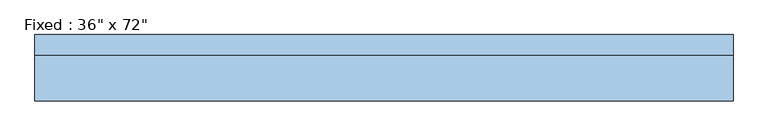
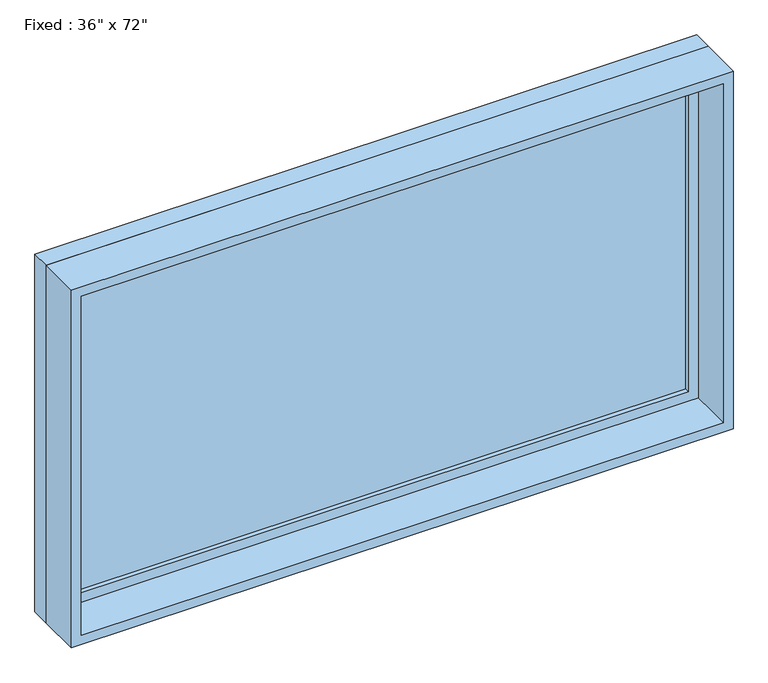
"""IFC4 building model written with IfcOpenShell, lengths in millimetres: window geometry."""

from ifc_helpers import new_model, si_unit, frame, origin, place, context, project, spatial, polyline, outline, extrude, source, transform, mapped, element, save


def window_a973ac2f(model_context):
    return source(origin(), model_context, "Body", "SweptSolid", [
        extrude(outline(polyline([(965.2, 53.975), (-1041.4, 53.975), (-1041.4, 66.675), (965.2, 66.675), (965.2, 53.975)])), frame((0.0, 0.0, 368.3), z_axis=(0.0, 0.0, 1.0), x_axis=(1.0, 0.0, 0.0)), (0.0, 0.0, 1.0), 1092.2),
        extrude(outline(polyline([(1504.95, -1085.85), (323.85, -1085.85), (323.85, 1009.65), (1504.95, 1009.65), (1504.95, -1085.85)]), holes=[polyline([(1460.5, -1041.4), (1460.5, 965.2), (368.3, 965.2), (368.3, -1041.4), (1460.5, -1041.4)])]), frame((0.0, 38.1, 0.0), z_axis=(0.0, 1.0, 0.0), x_axis=(0.0, 0.0, 1.0)), (0.0, 0.0, 1.0), 44.45),
        extrude(outline(polyline([(1524.0, -1104.9), (304.8, -1104.9), (304.8, 1028.7), (1524.0, 1028.7), (1524.0, -1104.9)]), holes=[polyline([(1492.25, -1073.15), (1492.25, 996.95), (336.55, 996.95), (336.55, -1073.15), (1492.25, -1073.15)])]), frame((0.0, -101.6, 0.0), z_axis=(0.0, 1.0, 0.0), x_axis=(0.0, 0.0, 1.0)), (0.0, 0.0, 1.0), 139.7),
        extrude(outline(polyline([(1524.0, 1028.7), (1524.0, -1104.9), (304.8, -1104.9), (304.8, 1028.7), (1524.0, 1028.7)]), holes=[polyline([(1504.95, 1009.65), (323.85, 1009.65), (323.85, -1085.85), (1504.95, -1085.85), (1504.95, 1009.65)])]), frame((0.0, 38.1, 0.0), z_axis=(0.0, 1.0, 0.0), x_axis=(0.0, 0.0, 1.0)), (0.0, 0.0, 1.0), 63.5),
    ])


if __name__ == "__main__":
    model = new_model("IFC4")
    model_context = context("Model", 3, world=origin())
    ifc_project = project(units=[si_unit("LENGTHUNIT", "METRE", prefix="MILLI")], contexts=[model_context])
    site = spatial("IfcSite", under=ifc_project)
    building = spatial("IfcBuilding", under=site)
    placement = place(None, origin())
    window_shape = window_a973ac2f(model_context)
    element("IfcWindow", 1, ObjectType="Fixed : 36\" x 72\"", at=placement, inside=building, context=model_context, shape_type="MappedRepresentation", body=[
        mapped(window_shape, transform((0.0, 0.0, 0.0), x_axis=(1.0, 0.0, 0.0), y_axis=(0.0, 1.0, 0.0), z_axis=(0.0, 0.0, 1.0))),
    ])
    save(model, "model.ifc")

# Revit data of these elements
# Type "Fixed : 36\" x 72\""
#   Type Mark = "9"
#   Construction Type Id = "GSP4R"
#   Assembly Code = "B2020100"
#   Analytic Construction = "1/8 in Pilkington single glazing"
#   Visual Light Transmittance = 0.9
#   Solar Heat Gain Coefficient = 0.78
#   Heat Transfer Coefficient (U) = 0.6496 BTU/(h·ft²·°F)
#   Height = 4' - 0"
#   Default Sill Height = 1' - 0"
#   Width = 7' - 0"
#   Window Inset = 0' - 0 3/4"
#   Define Thermal Properties by = 1
#   Glass Pane Material = Glass
#   Sash Material = Sash
#   Wall Closure = (empty or 0)
# Element 1 (IfcWindow, "Fixed : 36\" x 72\"")
#   Materials on its faces: "Sash", "Glass"
# Materials
#   "Glass": class "Glass", colour RGB 0 128 192, transparency 0.75, Description = "Soda Lime Glass", Cost = 0
#   "Sash": class "Wood", colour RGB 224 178 126, transparency 0
